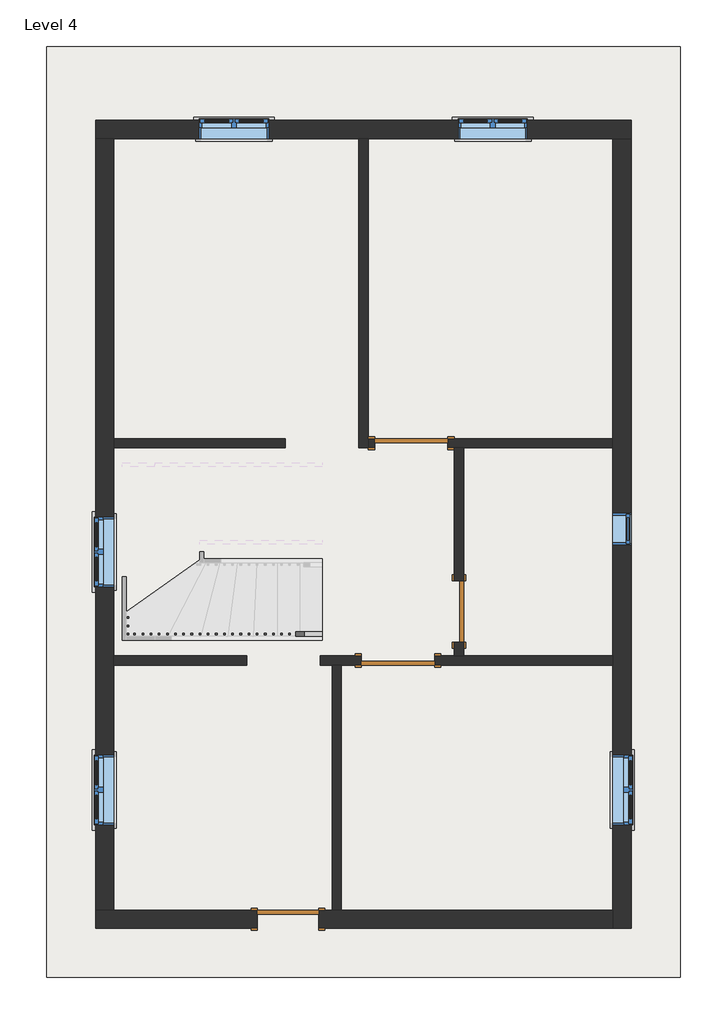
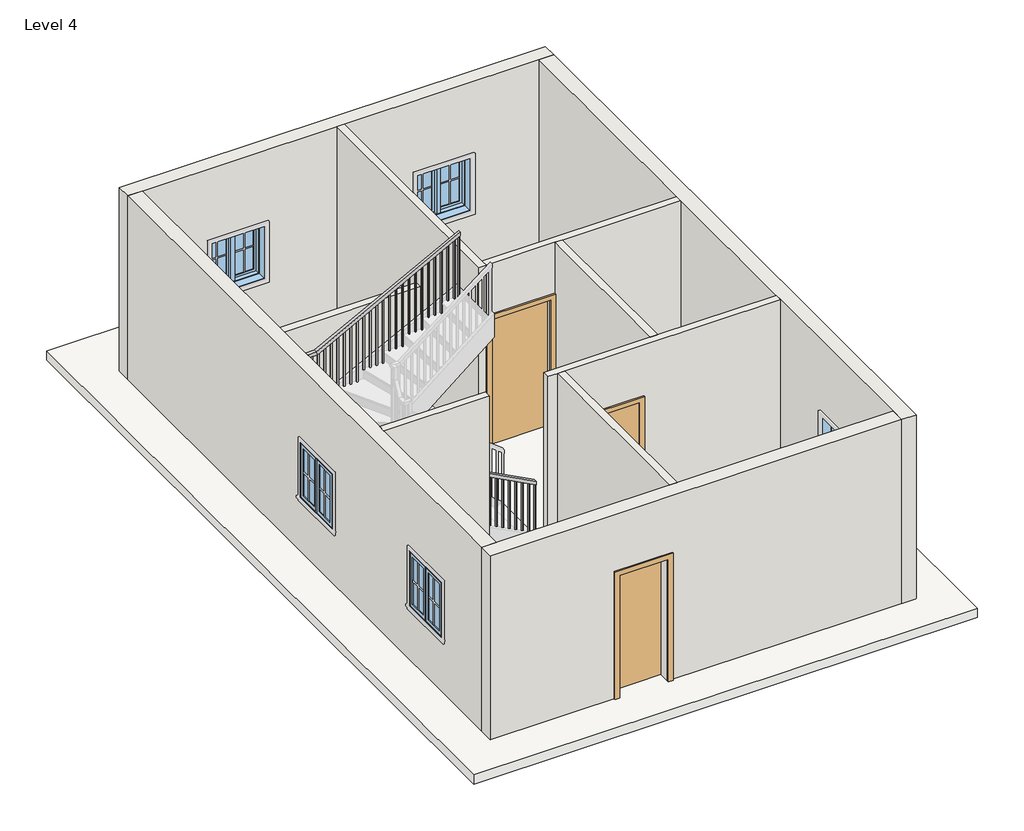
# One storey, part 1 of 2: 11 walls, 6 windows, 4 doors, 1 railing, 1 roof.
"""IFC4 building model written with IfcOpenShell, lengths in millimetres."""

from ifc_helpers import new_model, si_unit, frame, origin, place, context, project, spatial, polyline, outline, extrude, faceted_brep, transform, mapped, element, save
from components import door_d8f5dbb5, door_85036156, door_305aa2a5, door_e5f9f3c4, window_aa618e30, window_339605e1

model = new_model("IFC4")

# Units and contexts
model_context = context("Model", 3, world=origin())
ifc_project = project(units=[si_unit("LENGTHUNIT", "METRE", prefix="MILLI")], contexts=[model_context])

# Site, building, storey
site = spatial("IfcSite", under=ifc_project)
building = spatial("IfcBuilding", under=site)
storey = spatial("IfcBuildingStorey", under=building, Name="Level 4", Elevation=6400.8)

# Doors
placement = place(None, origin())
door_shape = door_d8f5dbb5(model_context)
element("IfcDoor", 1, ObjectType="Single-Flush : 30\" x 80\"", at=placement, inside=storey, context=model_context, shape_type="MappedRepresentation", body=[
    mapped(door_shape, transform((-82.2715692, -955.3070853, 6400.8), x_axis=(0.0, -1.0, 0.0), y_axis=(1.0, 0.0, 0.0), z_axis=(0.0, 0.0, 1.0))),
])
door_2_shape = door_85036156(model_context)
element("IfcDoor", 2, ObjectType="Single-Flush : 30\" x 80\"", at=placement, inside=storey, context=model_context, shape_type="MappedRepresentation", body=[
    mapped(door_2_shape, transform((-2212.5949167, -4784.3570853, 6400.8), x_axis=(-1.0, 0.0, 0.0), y_axis=(0.0, -1.0, 0.0), z_axis=(0.0, 0.0, 1.0))),
])
door_3_shape = door_305aa2a5(model_context)
element("IfcDoor", 3, ObjectType="Single-Flush : 36\" x 84\"", at=placement, inside=storey, context=model_context, shape_type="MappedRepresentation", body=[
    mapped(door_3_shape, transform((-677.5332429, 1140.1929147, 6400.8), x_axis=(-1.0, 0.0, 0.0), y_axis=(0.0, -1.0, 0.0), z_axis=(0.0, 0.0, 1.0))),
])
door_4_shape = door_e5f9f3c4(model_context)
element("IfcDoor", 4, ObjectType="Single-Flush : 36\" x 84\"", at=placement, inside=storey, context=model_context, shape_type="MappedRepresentation", body=[
    mapped(door_4_shape, transform((-842.6332429, -1564.9070853, 6400.8), x_axis=(-1.0, 0.0, 0.0), y_axis=(0.0, -1.0, 0.0), z_axis=(0.0, 0.0, 1.0))),
])

# Railing
element("IfcRailing", 5, ObjectType="Handrail - Rectangular", at=placement, inside=storey, context=model_context, shape_type="SolidModel", body=[
    faceted_brep([(-1783.4132248, -1260.1070853, 7484.5333333), (-1783.4132248, -1260.1070853, 7427.0742652), (-1783.4132248, -1209.3070853, 7427.0742652), (-1783.4132248, -1209.3070853, 7484.5333333), (-4041.1382869, -1260.1070853, 8677.8239201), (-4053.7373514, -1260.1070853, 8627.0239201), (-4053.7373514, -1209.3070853, 8627.0239201), (-4041.1382869, -1209.3070853, 8677.8239201), (-4225.5449167, -1260.1070853, 8677.8239201), (-4225.5449167, -1260.1070853, 8627.0239201), (-4174.7449167, -1209.3070853, 8627.0239201), (-4174.7449167, -1209.3070853, 8677.8239201), (-4225.5449167, -972.7952032, 8677.8239201), (-4225.5449167, -964.8446271, 8627.0239201), (-4174.7449167, -964.8446271, 8627.0239201), (-4174.7449167, -972.7952032, 8677.8239201), (-4225.5449167, 560.7810325, 9169.9094132), (-4225.5449167, 568.7316087, 9119.1094132), (-4174.7449167, 568.7316087, 9119.1094132), (-4174.7449167, 560.7810325, 9169.9094132), (-4225.5449167, 848.0929147, 9169.9094132), (-4225.5449167, 848.0929147, 9119.1094132), (-4174.7449167, 797.2929147, 9119.1094132), (-4174.7449167, 797.2929147, 9169.9094132), (-4041.1382869, 848.0929147, 9169.9094132), (-4028.5392223, 848.0929147, 9119.1094132), (-4028.5392223, 797.2929147, 9119.1094132), (-4041.1382869, 797.2929147, 9169.9094132), (-1783.4132248, 848.0929147, 10363.2), (-1783.4132248, 797.2929147, 10363.2), (-1783.4132248, 797.2929147, 10305.7409318), (-1783.4132248, 848.0929147, 10305.7409318)], [[[0, 1, 2, 3]], [[1, 0, 4, 5]], [[2, 1, 5, 6]], [[3, 2, 6, 7]], [[0, 3, 7, 4]], [[5, 4, 8, 9]], [[6, 5, 9, 10]], [[7, 6, 10, 11]], [[4, 7, 11, 8]], [[9, 8, 12, 13]], [[10, 9, 13, 14]], [[11, 10, 14, 15]], [[8, 11, 15, 12]], [[13, 12, 16, 17]], [[14, 13, 17, 18]], [[15, 14, 18, 19]], [[12, 15, 19, 16]], [[17, 16, 20, 21]], [[18, 17, 21, 22]], [[19, 18, 22, 23]], [[16, 19, 23, 20]], [[21, 20, 24, 25]], [[22, 21, 25, 26]], [[23, 22, 26, 27]], [[20, 23, 27, 24]], [[28, 29, 30, 31]], [[25, 24, 28, 31]], [[26, 25, 31, 30]], [[27, 26, 30, 29]], [[24, 27, 29, 28]]]),
    extrude(outline(polyline([(10258.4597858, -1872.8699167), (9279.4666667, -1872.8699167), (9279.4666667, -1853.8199167), (10268.5284102, -1853.8199167), (10258.4597858, -1872.8699167)])), frame((0.0, 813.1679147, 0.0), z_axis=(0.0, 1.0, 0.0), x_axis=(0.0, 0.0, 1.0)), (0.0, 0.0, 1.0), 19.05),
    extrude(outline(polyline([(10204.7604556, -1974.4699167), (9279.4666667, -1974.4699167), (9279.4666667, -1955.4199167), (10214.82908, -1955.4199167), (10204.7604556, -1974.4699167)])), frame((0.0, 813.1679147, 0.0), z_axis=(0.0, 1.0, 0.0), x_axis=(0.0, 0.0, 1.0)), (0.0, 0.0, 1.0), 19.05),
    extrude(outline(polyline([(10151.0611254, -2076.0699167), (9110.1333333, -2076.0699167), (9110.1333333, -2057.0199167), (10161.1297498, -2057.0199167), (10151.0611254, -2076.0699167)])), frame((0.0, 813.1679147, 0.0), z_axis=(0.0, 1.0, 0.0), x_axis=(0.0, 0.0, 1.0)), (0.0, 0.0, 1.0), 19.05),
    extrude(outline(polyline([(10097.3617952, -2177.6699167), (9110.1333333, -2177.6699167), (9110.1333333, -2158.6199167), (10107.4304196, -2158.6199167), (10097.3617952, -2177.6699167)])), frame((0.0, 813.1679147, 0.0), z_axis=(0.0, 1.0, 0.0), x_axis=(0.0, 0.0, 1.0)), (0.0, 0.0, 1.0), 19.05),
    extrude(outline(polyline([(10043.662465, -2279.2699167), (9110.1333333, -2279.2699167), (9110.1333333, -2260.2199167), (10053.7310894, -2260.2199167), (10043.662465, -2279.2699167)])), frame((0.0, 813.1679147, 0.0), z_axis=(0.0, 1.0, 0.0), x_axis=(0.0, 0.0, 1.0)), (0.0, 0.0, 1.0), 19.05),
    extrude(outline(polyline([(9989.9631348, -2380.8699167), (8940.8, -2380.8699167), (8940.8, -2361.8199167), (10000.0317592, -2361.8199167), (9989.9631348, -2380.8699167)])), frame((0.0, 813.1679147, 0.0), z_axis=(0.0, 1.0, 0.0), x_axis=(0.0, 0.0, 1.0)), (0.0, 0.0, 1.0), 19.05),
    extrude(outline(polyline([(9936.2638046, -2482.4699167), (8940.8, -2482.4699167), (8940.8, -2463.4199167), (9946.332429, -2463.4199167), (9936.2638046, -2482.4699167)])), frame((0.0, 813.1679147, 0.0), z_axis=(0.0, 1.0, 0.0), x_axis=(0.0, 0.0, 1.0)), (0.0, 0.0, 1.0), 19.05),
    extrude(outline(polyline([(9882.5644744, -2584.0699167), (8940.8, -2584.0699167), (8940.8, -2565.0199167), (9892.6330988, -2565.0199167), (9882.5644744, -2584.0699167)])), frame((0.0, 813.1679147, 0.0), z_axis=(0.0, 1.0, 0.0), x_axis=(0.0, 0.0, 1.0)), (0.0, 0.0, 1.0), 19.05),
    extrude(outline(polyline([(9828.8651442, -2685.6699167), (8771.4666667, -2685.6699167), (8771.4666667, -2666.6199167), (9838.9337686, -2666.6199167), (9828.8651442, -2685.6699167)])), frame((0.0, 813.1679147, 0.0), z_axis=(0.0, 1.0, 0.0), x_axis=(0.0, 0.0, 1.0)), (0.0, 0.0, 1.0), 19.05),
    extrude(outline(polyline([(9775.165814, -2787.2699167), (8771.4666667, -2787.2699167), (8771.4666667, -2768.2199167), (9785.2344384, -2768.2199167), (9775.165814, -2787.2699167)])), frame((0.0, 813.1679147, 0.0), z_axis=(0.0, 1.0, 0.0), x_axis=(0.0, 0.0, 1.0)), (0.0, 0.0, 1.0), 19.05),
    extrude(outline(polyline([(9721.4664838, -2888.8699167), (8771.4666667, -2888.8699167), (8771.4666667, -2869.8199167), (9731.5351082, -2869.8199167), (9721.4664838, -2888.8699167)])), frame((0.0, 813.1679147, 0.0), z_axis=(0.0, 1.0, 0.0), x_axis=(0.0, 0.0, 1.0)), (0.0, 0.0, 1.0), 19.05),
    extrude(outline(polyline([(9667.7671536, -2990.4699167), (8602.1333333, -2990.4699167), (8602.1333333, -2971.4199167), (9677.835778, -2971.4199167), (9667.7671536, -2990.4699167)])), frame((0.0, 813.1679147, 0.0), z_axis=(0.0, 1.0, 0.0), x_axis=(0.0, 0.0, 1.0)), (0.0, 0.0, 1.0), 19.05),
    extrude(outline(polyline([(9614.0678234, -3092.0699167), (8602.1333333, -3092.0699167), (8602.1333333, -3073.0199167), (9624.1364478, -3073.0199167), (9614.0678234, -3092.0699167)])), frame((0.0, 813.1679147, 0.0), z_axis=(0.0, 1.0, 0.0), x_axis=(0.0, 0.0, 1.0)), (0.0, 0.0, 1.0), 19.05),
    extrude(outline(polyline([(9560.3684932, -3193.6699167), (8602.1333333, -3193.6699167), (8602.1333333, -3174.6199167), (9570.4371176, -3174.6199167), (9560.3684932, -3193.6699167)])), frame((0.0, 813.1679147, 0.0), z_axis=(0.0, 1.0, 0.0), x_axis=(0.0, 0.0, 1.0)), (0.0, 0.0, 1.0), 19.05),
    extrude(outline(polyline([(9506.669163, -3295.2699167), (8602.1333333, -3295.2699167), (8602.1333333, -3276.2199167), (9516.7377874, -3276.2199167), (9506.669163, -3295.2699167)])), frame((0.0, 813.1679147, 0.0), z_axis=(0.0, 1.0, 0.0), x_axis=(0.0, 0.0, 1.0)), (0.0, 0.0, 1.0), 19.05),
    extrude(outline(polyline([(9452.9698328, -3396.8699167), (8432.8, -3396.8699167), (8432.8, -3377.8199167), (9463.0384572, -3377.8199167), (9452.9698328, -3396.8699167)])), frame((0.0, 813.1679147, 0.0), z_axis=(0.0, 1.0, 0.0), x_axis=(0.0, 0.0, 1.0)), (0.0, 0.0, 1.0), 19.05),
    extrude(outline(polyline([(9399.2705026, -3498.4699167), (8432.8, -3498.4699167), (8432.8, -3479.4199167), (9409.339127, -3479.4199167), (9399.2705026, -3498.4699167)])), frame((0.0, 813.1679147, 0.0), z_axis=(0.0, 1.0, 0.0), x_axis=(0.0, 0.0, 1.0)), (0.0, 0.0, 1.0), 19.05),
    extrude(outline(polyline([(9345.5711724, -3600.0699167), (8432.8, -3600.0699167), (8432.8, -3581.0199167), (9355.6397968, -3581.0199167), (9345.5711724, -3600.0699167)])), frame((0.0, 813.1679147, 0.0), z_axis=(0.0, 1.0, 0.0), x_axis=(0.0, 0.0, 1.0)), (0.0, 0.0, 1.0), 19.05),
    extrude(outline(polyline([(9291.8718422, -3701.6699167), (8432.8, -3701.6699167), (8432.8, -3682.6199167), (9301.9404666, -3682.6199167), (9291.8718422, -3701.6699167)])), frame((0.0, 813.1679147, 0.0), z_axis=(0.0, 1.0, 0.0), x_axis=(0.0, 0.0, 1.0)), (0.0, 0.0, 1.0), 19.05),
    extrude(outline(polyline([(9238.172512, -3803.2699167), (8263.4666667, -3803.2699167), (8263.4666667, -3784.2199167), (9248.2411364, -3784.2199167), (9238.172512, -3803.2699167)])), frame((0.0, 813.1679147, 0.0), z_axis=(0.0, 1.0, 0.0), x_axis=(0.0, 0.0, 1.0)), (0.0, 0.0, 1.0), 19.05),
    extrude(outline(polyline([(9184.4731818, -3904.8699167), (8263.4666667, -3904.8699167), (8263.4666667, -3885.8199167), (9194.5418062, -3885.8199167), (9184.4731818, -3904.8699167)])), frame((0.0, 813.1679147, 0.0), z_axis=(0.0, 1.0, 0.0), x_axis=(0.0, 0.0, 1.0)), (0.0, 0.0, 1.0), 19.05),
    extrude(outline(polyline([(9130.7738516, -4006.4699167), (8263.4666667, -4006.4699167), (8263.4666667, -3987.4199167), (9140.842476, -3987.4199167), (9130.7738516, -4006.4699167)])), frame((0.0, 813.1679147, 0.0), z_axis=(0.0, 1.0, 0.0), x_axis=(0.0, 0.0, 1.0)), (0.0, 0.0, 1.0), 19.05),
    extrude(outline(polyline([(-4108.0699167, 832.2179147), (-4089.0199167, 832.2179147), (-4089.0199167, 813.1679147), (-4108.0699167, 813.1679147), (-4108.0699167, 832.2179147)])), frame((0.0, 0.0, 8263.4666667), z_axis=(0.0, 0.0, 1.0), x_axis=(1.0, 0.0, 0.0)), (0.0, 0.0, 1.0), 855.6427466),
    extrude(outline(polyline([(-4209.6699167, 787.7679147), (-4209.6699167, 806.8179147), (-4190.6199167, 806.8179147), (-4190.6199167, 787.7679147), (-4209.6699167, 787.7679147)])), frame((0.0, 0.0, 8263.4666667), z_axis=(0.0, 0.0, 1.0), x_axis=(1.0, 0.0, 0.0)), (0.0, 0.0, 1.0), 855.6427466),
    extrude(outline(polyline([(-4209.6699167, 686.1679147), (-4209.6699167, 705.2179147), (-4190.6199167, 705.2179147), (-4190.6199167, 686.1679147), (-4209.6699167, 686.1679147)])), frame((0.0, 0.0, 8263.4666667), z_axis=(0.0, 0.0, 1.0), x_axis=(1.0, 0.0, 0.0)), (0.0, 0.0, 1.0), 855.6427466),
    extrude(outline(polyline([(-4209.6699167, 584.5679147), (-4209.6699167, 603.6179147), (-4190.6199167, 603.6179147), (-4190.6199167, 584.5679147), (-4209.6699167, 584.5679147)])), frame((0.0, 0.0, 8263.4666667), z_axis=(0.0, 0.0, 1.0), x_axis=(1.0, 0.0, 0.0)), (0.0, 0.0, 1.0), 855.6427466),
    extrude(outline(polyline([(502.0179147, 9097.7026907), (502.0179147, 8094.1333333), (482.9679147, 8094.1333333), (482.9679147, 9091.5900316), (502.0179147, 9097.7026907)])), frame((-4209.6699167, 0.0, 0.0), z_axis=(1.0, 0.0, 0.0), x_axis=(0.0, 1.0, 0.0)), (0.0, 0.0, 1.0), 19.05),
    extrude(outline(polyline([(400.4179147, 9065.1018425), (400.4179147, 8094.1333333), (381.3679147, 8094.1333333), (381.3679147, 9058.9891834), (400.4179147, 9065.1018425)])), frame((-4209.6699167, 0.0, 0.0), z_axis=(1.0, 0.0, 0.0), x_axis=(0.0, 1.0, 0.0)), (0.0, 0.0, 1.0), 19.05),
    extrude(outline(polyline([(298.8179147, 9032.5009942), (298.8179147, 8094.1333333), (279.7679147, 8094.1333333), (279.7679147, 9026.3883352), (298.8179147, 9032.5009942)])), frame((-4209.6699167, 0.0, 0.0), z_axis=(1.0, 0.0, 0.0), x_axis=(0.0, 1.0, 0.0)), (0.0, 0.0, 1.0), 19.05),
    extrude(outline(polyline([(197.2179147, 8999.900146), (197.2179147, 8094.1333333), (178.1679147, 8094.1333333), (178.1679147, 8993.787487), (197.2179147, 8999.900146)])), frame((-4209.6699167, 0.0, 0.0), z_axis=(1.0, 0.0, 0.0), x_axis=(0.0, 1.0, 0.0)), (0.0, 0.0, 1.0), 19.05),
    extrude(outline(polyline([(95.6179147, 8967.2992978), (95.6179147, 8094.1333333), (76.5679147, 8094.1333333), (76.5679147, 8961.1866387), (95.6179147, 8967.2992978)])), frame((-4209.6699167, 0.0, 0.0), z_axis=(1.0, 0.0, 0.0), x_axis=(0.0, 1.0, 0.0)), (0.0, 0.0, 1.0), 19.05),
    extrude(outline(polyline([(-5.9820853, 8934.6984495), (-5.9820853, 7924.8), (-25.0320853, 7924.8), (-25.0320853, 8928.5857905), (-5.9820853, 8934.6984495)])), frame((-4209.6699167, 0.0, 0.0), z_axis=(1.0, 0.0, 0.0), x_axis=(0.0, 1.0, 0.0)), (0.0, 0.0, 1.0), 19.05),
    extrude(outline(polyline([(-107.5820853, 8902.0976013), (-107.5820853, 7924.8), (-126.6320853, 7924.8), (-126.6320853, 8895.9849423), (-107.5820853, 8902.0976013)])), frame((-4209.6699167, 0.0, 0.0), z_axis=(1.0, 0.0, 0.0), x_axis=(0.0, 1.0, 0.0)), (0.0, 0.0, 1.0), 19.05),
    extrude(outline(polyline([(-209.1820853, 8869.4967531), (-209.1820853, 7924.8), (-228.2320853, 7924.8), (-228.2320853, 8863.384094), (-209.1820853, 8869.4967531)])), frame((-4209.6699167, 0.0, 0.0), z_axis=(1.0, 0.0, 0.0), x_axis=(0.0, 1.0, 0.0)), (0.0, 0.0, 1.0), 19.05),
    extrude(outline(polyline([(-310.7820853, 8836.8959049), (-310.7820853, 7924.8), (-329.8320853, 7924.8), (-329.8320853, 8830.7832458), (-310.7820853, 8836.8959049)])), frame((-4209.6699167, 0.0, 0.0), z_axis=(1.0, 0.0, 0.0), x_axis=(0.0, 1.0, 0.0)), (0.0, 0.0, 1.0), 19.05),
    extrude(outline(polyline([(-412.3820853, 8804.2950566), (-412.3820853, 7924.8), (-431.4320853, 7924.8), (-431.4320853, 8798.1823976), (-412.3820853, 8804.2950566)])), frame((-4209.6699167, 0.0, 0.0), z_axis=(1.0, 0.0, 0.0), x_axis=(0.0, 1.0, 0.0)), (0.0, 0.0, 1.0), 19.05),
    extrude(outline(polyline([(-513.9820853, 8771.6942084), (-513.9820853, 7755.4666667), (-533.0320853, 7755.4666667), (-533.0320853, 8765.5815494), (-513.9820853, 8771.6942084)])), frame((-4209.6699167, 0.0, 0.0), z_axis=(1.0, 0.0, 0.0), x_axis=(0.0, 1.0, 0.0)), (0.0, 0.0, 1.0), 19.05),
    extrude(outline(polyline([(-615.5820853, 8739.0933602), (-615.5820853, 7755.4666667), (-634.6320853, 7755.4666667), (-634.6320853, 8732.9807011), (-615.5820853, 8739.0933602)])), frame((-4209.6699167, 0.0, 0.0), z_axis=(1.0, 0.0, 0.0), x_axis=(0.0, 1.0, 0.0)), (0.0, 0.0, 1.0), 19.05),
    extrude(outline(polyline([(-717.1820853, 8706.492512), (-717.1820853, 7755.4666667), (-736.2320853, 7755.4666667), (-736.2320853, 8700.3798529), (-717.1820853, 8706.492512)])), frame((-4209.6699167, 0.0, 0.0), z_axis=(1.0, 0.0, 0.0), x_axis=(0.0, 1.0, 0.0)), (0.0, 0.0, 1.0), 19.05),
    extrude(outline(polyline([(-818.7820853, 8673.8916637), (-818.7820853, 7755.4666667), (-837.8320853, 7755.4666667), (-837.8320853, 8667.7790047), (-818.7820853, 8673.8916637)])), frame((-4209.6699167, 0.0, 0.0), z_axis=(1.0, 0.0, 0.0), x_axis=(0.0, 1.0, 0.0)), (0.0, 0.0, 1.0), 19.05),
    extrude(outline(polyline([(-920.3820853, 8641.2908155), (-920.3820853, 7755.4666667), (-939.4320853, 7755.4666667), (-939.4320853, 8635.1781565), (-920.3820853, 8641.2908155)])), frame((-4209.6699167, 0.0, 0.0), z_axis=(1.0, 0.0, 0.0), x_axis=(0.0, 1.0, 0.0)), (0.0, 0.0, 1.0), 19.05),
    extrude(outline(polyline([(-4209.6699167, -1041.0320853), (-4209.6699167, -1021.9820853), (-4190.6199167, -1021.9820853), (-4190.6199167, -1041.0320853), (-4209.6699167, -1041.0320853)])), frame((0.0, 0.0, 7586.1333333), z_axis=(0.0, 0.0, 1.0), x_axis=(1.0, 0.0, 0.0)), (0.0, 0.0, 1.0), 1040.8905868),
    extrude(outline(polyline([(-4209.6699167, -1142.6320853), (-4209.6699167, -1123.5820853), (-4190.6199167, -1123.5820853), (-4190.6199167, -1142.6320853), (-4209.6699167, -1142.6320853)])), frame((0.0, 0.0, 7586.1333333), z_axis=(0.0, 0.0, 1.0), x_axis=(1.0, 0.0, 0.0)), (0.0, 0.0, 1.0), 1040.8905868),
    extrude(outline(polyline([(-4110.6882248, -1244.2320853), (-4129.7382248, -1244.2320853), (-4129.7382248, -1225.1820853), (-4110.6882248, -1225.1820853), (-4110.6882248, -1244.2320853)])), frame((0.0, 0.0, 7586.1333333), z_axis=(0.0, 0.0, 1.0), x_axis=(1.0, 0.0, 0.0)), (0.0, 0.0, 1.0), 1040.8905868),
    extrude(outline(polyline([(8613.4938418, -4028.1382248), (7586.1333333, -4028.1382248), (7586.1333333, -4009.0882248), (8603.4252174, -4009.0882248), (8613.4938418, -4028.1382248)])), frame((0.0, -1244.2320853, 0.0), z_axis=(0.0, 1.0, 0.0), x_axis=(0.0, 0.0, 1.0)), (0.0, 0.0, 1.0), 19.05),
    extrude(outline(polyline([(8559.7945116, -3926.5382248), (7586.1333333, -3926.5382248), (7586.1333333, -3907.4882248), (8549.7258872, -3907.4882248), (8559.7945116, -3926.5382248)])), frame((0.0, -1244.2320853, 0.0), z_axis=(0.0, 1.0, 0.0), x_axis=(0.0, 0.0, 1.0)), (0.0, 0.0, 1.0), 19.05),
    extrude(outline(polyline([(8506.0951814, -3824.9382248), (7586.1333333, -3824.9382248), (7586.1333333, -3805.8882248), (8496.026557, -3805.8882248), (8506.0951814, -3824.9382248)])), frame((0.0, -1244.2320853, 0.0), z_axis=(0.0, 1.0, 0.0), x_axis=(0.0, 0.0, 1.0)), (0.0, 0.0, 1.0), 19.05),
    extrude(outline(polyline([(8452.3958512, -3723.3382248), (7586.1333333, -3723.3382248), (7586.1333333, -3704.2882248), (8442.3272268, -3704.2882248), (8452.3958512, -3723.3382248)])), frame((0.0, -1244.2320853, 0.0), z_axis=(0.0, 1.0, 0.0), x_axis=(0.0, 0.0, 1.0)), (0.0, 0.0, 1.0), 19.05),
    extrude(outline(polyline([(8398.696521, -3621.7382248), (7416.8, -3621.7382248), (7416.8, -3602.6882248), (8388.6278966, -3602.6882248), (8398.696521, -3621.7382248)])), frame((0.0, -1244.2320853, 0.0), z_axis=(0.0, 1.0, 0.0), x_axis=(0.0, 0.0, 1.0)), (0.0, 0.0, 1.0), 19.05),
    extrude(outline(polyline([(8344.9971908, -3520.1382248), (7416.8, -3520.1382248), (7416.8, -3501.0882248), (8334.9285664, -3501.0882248), (8344.9971908, -3520.1382248)])), frame((0.0, -1244.2320853, 0.0), z_axis=(0.0, 1.0, 0.0), x_axis=(0.0, 0.0, 1.0)), (0.0, 0.0, 1.0), 19.05),
    extrude(outline(polyline([(8291.2978606, -3418.5382248), (7416.8, -3418.5382248), (7416.8, -3399.4882248), (8281.2292362, -3399.4882248), (8291.2978606, -3418.5382248)])), frame((0.0, -1244.2320853, 0.0), z_axis=(0.0, 1.0, 0.0), x_axis=(0.0, 0.0, 1.0)), (0.0, 0.0, 1.0), 19.05),
    extrude(outline(polyline([(8237.5985304, -3316.9382248), (7416.8, -3316.9382248), (7416.8, -3297.8882248), (8227.529906, -3297.8882248), (8237.5985304, -3316.9382248)])), frame((0.0, -1244.2320853, 0.0), z_axis=(0.0, 1.0, 0.0), x_axis=(0.0, 0.0, 1.0)), (0.0, 0.0, 1.0), 19.05),
    extrude(outline(polyline([(8183.8992002, -3215.3382248), (7247.4666667, -3215.3382248), (7247.4666667, -3196.2882248), (8173.8305758, -3196.2882248), (8183.8992002, -3215.3382248)])), frame((0.0, -1244.2320853, 0.0), z_axis=(0.0, 1.0, 0.0), x_axis=(0.0, 0.0, 1.0)), (0.0, 0.0, 1.0), 19.05),
    extrude(outline(polyline([(8130.19987, -3113.7382248), (7247.4666667, -3113.7382248), (7247.4666667, -3094.6882248), (8120.1312456, -3094.6882248), (8130.19987, -3113.7382248)])), frame((0.0, -1244.2320853, 0.0), z_axis=(0.0, 1.0, 0.0), x_axis=(0.0, 0.0, 1.0)), (0.0, 0.0, 1.0), 19.05),
    extrude(outline(polyline([(8076.5005398, -3012.1382248), (7247.4666667, -3012.1382248), (7247.4666667, -2993.0882248), (8066.4319154, -2993.0882248), (8076.5005398, -3012.1382248)])), frame((0.0, -1244.2320853, 0.0), z_axis=(0.0, 1.0, 0.0), x_axis=(0.0, 0.0, 1.0)), (0.0, 0.0, 1.0), 19.05),
    extrude(outline(polyline([(8022.8012096, -2910.5382248), (7078.1333333, -2910.5382248), (7078.1333333, -2891.4882248), (8012.7325852, -2891.4882248), (8022.8012096, -2910.5382248)])), frame((0.0, -1244.2320853, 0.0), z_axis=(0.0, 1.0, 0.0), x_axis=(0.0, 0.0, 1.0)), (0.0, 0.0, 1.0), 19.05),
    extrude(outline(polyline([(7969.1018794, -2808.9382248), (7078.1333333, -2808.9382248), (7078.1333333, -2789.8882248), (7959.033255, -2789.8882248), (7969.1018794, -2808.9382248)])), frame((0.0, -1244.2320853, 0.0), z_axis=(0.0, 1.0, 0.0), x_axis=(0.0, 0.0, 1.0)), (0.0, 0.0, 1.0), 19.05),
    extrude(outline(polyline([(7915.4025492, -2707.3382248), (7078.1333333, -2707.3382248), (7078.1333333, -2688.2882248), (7905.3339248, -2688.2882248), (7915.4025492, -2707.3382248)])), frame((0.0, -1244.2320853, 0.0), z_axis=(0.0, 1.0, 0.0), x_axis=(0.0, 0.0, 1.0)), (0.0, 0.0, 1.0), 19.05),
    extrude(outline(polyline([(7861.703219, -2605.7382248), (6908.8, -2605.7382248), (6908.8, -2586.6882248), (7851.6345946, -2586.6882248), (7861.703219, -2605.7382248)])), frame((0.0, -1244.2320853, 0.0), z_axis=(0.0, 1.0, 0.0), x_axis=(0.0, 0.0, 1.0)), (0.0, 0.0, 1.0), 19.05),
    extrude(outline(polyline([(7808.0038888, -2504.1382248), (6908.8, -2504.1382248), (6908.8, -2485.0882248), (7797.9352644, -2485.0882248), (7808.0038888, -2504.1382248)])), frame((0.0, -1244.2320853, 0.0), z_axis=(0.0, 1.0, 0.0), x_axis=(0.0, 0.0, 1.0)), (0.0, 0.0, 1.0), 19.05),
    extrude(outline(polyline([(7754.3045586, -2402.5382248), (6908.8, -2402.5382248), (6908.8, -2383.4882248), (7744.2359342, -2383.4882248), (7754.3045586, -2402.5382248)])), frame((0.0, -1244.2320853, 0.0), z_axis=(0.0, 1.0, 0.0), x_axis=(0.0, 0.0, 1.0)), (0.0, 0.0, 1.0), 19.05),
    extrude(outline(polyline([(7700.6052284, -2300.9382248), (6739.4666667, -2300.9382248), (6739.4666667, -2281.8882248), (7690.536604, -2281.8882248), (7700.6052284, -2300.9382248)])), frame((0.0, -1244.2320853, 0.0), z_axis=(0.0, 1.0, 0.0), x_axis=(0.0, 0.0, 1.0)), (0.0, 0.0, 1.0), 19.05),
    extrude(outline(polyline([(7646.9058982, -2199.3382248), (6739.4666667, -2199.3382248), (6739.4666667, -2180.2882248), (7636.8372738, -2180.2882248), (7646.9058982, -2199.3382248)])), frame((0.0, -1244.2320853, 0.0), z_axis=(0.0, 1.0, 0.0), x_axis=(0.0, 0.0, 1.0)), (0.0, 0.0, 1.0), 19.05),
    extrude(outline(polyline([(7593.206568, -2097.7382248), (6739.4666667, -2097.7382248), (6739.4666667, -2078.6882248), (7583.1379436, -2078.6882248), (7593.206568, -2097.7382248)])), frame((0.0, -1244.2320853, 0.0), z_axis=(0.0, 1.0, 0.0), x_axis=(0.0, 0.0, 1.0)), (0.0, 0.0, 1.0), 19.05),
    extrude(outline(polyline([(7539.5072378, -1996.1382248), (6570.1333333, -1996.1382248), (6570.1333333, -1977.0882248), (7529.4386134, -1977.0882248), (7539.5072378, -1996.1382248)])), frame((0.0, -1244.2320853, 0.0), z_axis=(0.0, 1.0, 0.0), x_axis=(0.0, 0.0, 1.0)), (0.0, 0.0, 1.0), 19.05),
    extrude(outline(polyline([(7485.8079076, -1894.5382248), (6570.1333333, -1894.5382248), (6570.1333333, -1875.4882248), (7475.7392831, -1875.4882248), (7485.8079076, -1894.5382248)])), frame((0.0, -1244.2320853, 0.0), z_axis=(0.0, 1.0, 0.0), x_axis=(0.0, 0.0, 1.0)), (0.0, 0.0, 1.0), 19.05),
    extrude(outline(polyline([(-4209.6699167, 813.1679147), (-4209.6699167, 832.2179147), (-4190.6199167, 832.2179147), (-4190.6199167, 813.1679147), (-4209.6699167, 813.1679147)])), frame((0.0, 0.0, 8263.4666667), z_axis=(0.0, 0.0, 1.0), x_axis=(1.0, 0.0, 0.0)), (0.0, 0.0, 1.0), 855.6427466),
    extrude(outline(polyline([(-4190.6199167, -1244.2320853), (-4209.6699167, -1244.2320853), (-4209.6699167, -1225.1820853), (-4190.6199167, -1225.1820853), (-4190.6199167, -1244.2320853)])), frame((0.0, 0.0, 7586.1333333), z_axis=(0.0, 0.0, 1.0), x_axis=(1.0, 0.0, 0.0)), (0.0, 0.0, 1.0), 1040.8905868),
    extrude(outline(polyline([(10295.6723074, -1802.4632248), (9279.4666667, -1802.4632248), (9279.4666667, -1783.4132248), (10305.7409318, -1783.4132248), (10295.6723074, -1802.4632248)])), frame((0.0, 813.1679147, 0.0), z_axis=(0.0, 1.0, 0.0), x_axis=(0.0, 0.0, 1.0)), (0.0, 0.0, 1.0), 19.05),
    extrude(outline(polyline([(7437.1428896, -1802.4632248), (6570.1333333, -1802.4632248), (6570.1333333, -1783.4132248), (7427.0742652, -1783.4132248), (7437.1428896, -1802.4632248)])), frame((0.0, -1244.2320853, 0.0), z_axis=(0.0, 1.0, 0.0), x_axis=(0.0, 0.0, 1.0)), (0.0, 0.0, 1.0), 19.05),
])

# Roof
element("IfcRoof", 6, ObjectType="Generic - 12\"", at=placement, inside=storey, context=model_context, shape_type="SweptSolid", body=[
    extrude(outline(polyline([(-5216.1449167, 6076.3773594), (2670.5550833, 6076.3773594), (2670.5550833, -5508.2570853), (-5216.1449167, -5508.2570853), (-5216.1449167, 6076.3773594)])), frame((0.0, 0.0, 6248.4), z_axis=(0.0, 0.0, 1.0), x_axis=(1.0, 0.0, 0.0)), (0.0, 0.0, 1.0), 152.4),
])

# Walls
element("IfcWall", 7, ObjectType="WALL4.5\"", at=placement, inside=storey, context=model_context, shape_type="Brep", body=[
    faceted_brep([(-1329.9449167, 4931.1429147, 6400.8), (-1329.9449167, 1083.0429147, 6400.8), (-1329.9449167, 1083.0429147, 9448.8), (-1329.9449167, 4931.1429147, 9448.8), (-1215.6449167, 4931.1429147, 6400.8), (-1215.6449167, 4931.1429147, 9448.8), (-1215.6449167, 1197.3429147, 9448.8), (-1215.6449167, 1083.0429147, 9448.8), (-1215.6449167, 1083.0429147, 6400.8), (-1215.6449167, 1197.3429147, 6400.8)], [[[0, 1, 2, 3]], [[4, 5, 6, 7, 8, 9]], [[1, 0, 4, 9, 8]], [[0, 3, 5, 4]], [[2, 1, 8, 7]], [[3, 2, 7, 6, 5]]]),
])
element("IfcWall", 8, ObjectType="WALL4.5\"", at=placement, inside=storey, context=model_context, shape_type="Brep", body=[
    faceted_brep([(-1215.6449167, 1083.0429147, 6400.8), (-1134.7332429, 1083.0429147, 6400.8), (-1134.7332429, 1083.0429147, 8534.4), (-220.3332429, 1083.0429147, 8534.4), (-220.3332429, 1083.0429147, 6400.8), (-139.4215692, 1083.0429147, 6400.8), (-25.1215692, 1083.0429147, 6400.8), (1832.3550833, 1083.0429147, 6400.8), (1832.3550833, 1083.0429147, 9448.8), (-25.1215692, 1083.0429147, 9448.8), (-139.4215692, 1083.0429147, 9448.8), (-1215.6449167, 1083.0429147, 9448.8), (-1134.7332429, 1197.3429147, 8534.4), (-1134.7332429, 1197.3429147, 6400.8), (-1215.6449167, 1197.3429147, 6400.8), (-1215.6449167, 1197.3429147, 9448.8), (1832.3550833, 1197.3429147, 9448.8), (1832.3550833, 1197.3429147, 6400.8), (-220.3332429, 1197.3429147, 6400.8), (-220.3332429, 1197.3429147, 8534.4)], [[[0, 1, 2, 3, 4, 5, 6, 7, 8, 9, 10, 11]], [[12, 13, 14, 15, 16, 17, 18, 19]], [[18, 17, 7, 6, 5, 4]], [[14, 13, 1, 0]], [[0, 11, 15, 14]], [[8, 7, 17, 16]], [[2, 1, 13, 12]], [[3, 2, 12, 19]], [[4, 3, 19, 18]], [[11, 10, 9, 8, 16, 15]]]),
])
element("IfcWall", 9, ObjectType="WALL4.5\"", at=placement, inside=storey, context=model_context, shape_type="SweptSolid", body=[
    extrude(outline(polyline([(-2244.3449167, 1083.0429147), (-4377.9449167, 1083.0429147), (-4377.9449167, 1197.3429147), (-2244.3449167, 1197.3429147), (-2244.3449167, 1083.0429147)])), frame((0.0, 0.0, 6400.8), z_axis=(0.0, 0.0, 1.0), x_axis=(1.0, 0.0, 0.0)), (0.0, 0.0, 1.0), 3048.0),
])
element("IfcWall", 10, ObjectType="WALL4.5\"", at=placement, inside=storey, context=model_context, shape_type="SweptSolid", body=[
    extrude(outline(polyline([(-1336.3070853, 8432.8), (-1336.3070853, 6400.8), (-1507.7570853, 6400.8), (-1507.7570853, 9448.8), (1083.0429147, 9448.8), (1083.0429147, 6400.8), (-574.3070853, 6400.8), (-574.3070853, 8432.8), (-1336.3070853, 8432.8)])), frame((-139.4215692, 0.0, 0.0), z_axis=(1.0, 0.0, 0.0), x_axis=(0.0, 1.0, 0.0)), (0.0, 0.0, 1.0), 114.3),
])
element("IfcWall", 11, ObjectType="WALL4.5\"", at=placement, inside=storey, context=model_context, shape_type="SweptSolid", body=[
    extrude(outline(polyline([(-2726.9449167, -1622.0570853), (-4377.9449167, -1622.0570853), (-4377.9449167, -1507.7570853), (-2726.9449167, -1507.7570853), (-2726.9449167, -1622.0570853)])), frame((0.0, 0.0, 6400.8), z_axis=(0.0, 0.0, 1.0), x_axis=(1.0, 0.0, 0.0)), (0.0, 0.0, 1.0), 3048.0),
])
element("IfcWall", 12, ObjectType="WALL4.5\"", at=placement, inside=storey, context=model_context, shape_type="Brep", body=[
    faceted_brep([(-1812.5449167, -1622.0570853, 6400.8), (-1660.1449167, -1622.0570853, 6400.8), (-1545.8449167, -1622.0570853, 6400.8), (-1299.8332429, -1622.0570853, 6400.8), (-1299.8332429, -1622.0570853, 8534.4), (-385.4332429, -1622.0570853, 8534.4), (-385.4332429, -1622.0570853, 6400.8), (1832.3550833, -1622.0570853, 6400.8), (1832.3550833, -1622.0570853, 9448.8), (-1545.8449167, -1622.0570853, 9448.8), (-1660.1449167, -1622.0570853, 9448.8), (-1812.5449167, -1622.0570853, 9448.8), (-1299.8332429, -1507.7570853, 8534.4), (-1299.8332429, -1507.7570853, 6400.8), (-1812.5449167, -1507.7570853, 6400.8), (-1812.5449167, -1507.7570853, 9448.8), (-139.4215692, -1507.7570853, 9448.8), (-25.1215692, -1507.7570853, 9448.8), (1832.3550833, -1507.7570853, 9448.8), (1832.3550833, -1507.7570853, 6400.8), (-25.1215692, -1507.7570853, 6400.8), (-139.4215692, -1507.7570853, 6400.8), (-385.4332429, -1507.7570853, 6400.8), (-385.4332429, -1507.7570853, 8534.4)], [[[0, 1, 2, 3, 4, 5, 6, 7, 8, 9, 10, 11]], [[12, 13, 14, 15, 16, 17, 18, 19, 20, 21, 22, 23]], [[14, 13, 3, 2, 1, 0]], [[22, 21, 20, 19, 7, 6]], [[0, 11, 15, 14]], [[8, 7, 19, 18]], [[4, 3, 13, 12]], [[5, 4, 12, 23]], [[6, 5, 23, 22]], [[11, 10, 9, 8, 18, 17, 16, 15]]]),
])
element("IfcWall", 13, ObjectType="WALL4.5\"", at=placement, inside=storey, context=model_context, shape_type="SweptSolid", body=[
    extrude(outline(polyline([(-1660.1449167, -4670.0570853), (-1660.1449167, -1622.0570853), (-1545.8449167, -1622.0570853), (-1545.8449167, -4670.0570853), (-1660.1449167, -4670.0570853)])), frame((0.0, 0.0, 6400.8), z_axis=(0.0, 0.0, 1.0), x_axis=(1.0, 0.0, 0.0)), (0.0, 0.0, 1.0), 3048.0),
])
element("IfcWall", 14, ObjectType="WALL9\"", at=placement, inside=storey, context=model_context, shape_type="Brep", body=[
    faceted_brep([(-4606.5449167, 4931.1429147, 6400.8), (-4377.9449167, 4931.1429147, 6400.8), (-1329.9449167, 4931.1429147, 6400.8), (-1215.6449167, 4931.1429147, 6400.8), (1832.3550833, 4931.1429147, 6400.8), (2060.9550833, 4931.1429147, 6400.8), (2060.9550833, 4931.1429147, 9448.8), (1832.3550833, 4931.1429147, 9448.8), (-1215.6449167, 4931.1429147, 9448.8), (-1329.9449167, 4931.1429147, 9448.8), (-4377.9449167, 4931.1429147, 9448.8), (-4606.5449167, 4931.1429147, 9448.8), (-2450.7199167, 4931.1429147, 8229.6), (-2450.7199167, 4931.1429147, 7315.2), (-3314.3199167, 4931.1429147, 7315.2), (-3314.3199167, 4931.1429147, 8229.6), (768.7300833, 4931.1429147, 8229.6), (768.7300833, 4931.1429147, 7315.2), (-94.8699167, 4931.1429147, 7315.2), (-94.8699167, 4931.1429147, 8229.6), (-4606.5449167, 5159.7429147, 6400.8), (-4606.5449167, 5159.7429147, 9448.8), (2060.9550833, 5159.7429147, 9448.8), (2060.9550833, 5159.7429147, 6400.8), (-2450.7199167, 5159.7429147, 8229.6), (-3314.3199167, 5159.7429147, 8229.6), (-3314.3199167, 5159.7429147, 7315.2), (-2450.7199167, 5159.7429147, 7315.2), (768.7300833, 5159.7429147, 8229.6), (-94.8699167, 5159.7429147, 8229.6), (-94.8699167, 5159.7429147, 7315.2), (768.7300833, 5159.7429147, 7315.2)], [[[0, 1, 2, 3, 4, 5, 6, 7, 8, 9, 10, 11], [12, 13, 14, 15], [16, 17, 18, 19]], [[20, 21, 22, 23], [24, 25, 26, 27], [28, 29, 30, 31]], [[5, 4, 3, 2, 1, 0, 20, 23]], [[6, 5, 23, 22]], [[0, 11, 21, 20]], [[13, 12, 24, 27]], [[14, 13, 27, 26]], [[15, 14, 26, 25]], [[12, 15, 25, 24]], [[17, 16, 28, 31]], [[18, 17, 31, 30]], [[19, 18, 30, 29]], [[16, 19, 29, 28]], [[11, 10, 9, 8, 7, 6, 22, 21]]]),
])
element("IfcWall", 15, ObjectType="WALL9\"", at=placement, inside=storey, context=model_context, shape_type="Brep", body=[
    faceted_brep([(1832.3550833, 4931.1429147, 6400.8), (1832.3550833, 1197.3429147, 6400.8), (1832.3550833, 1083.0429147, 6400.8), (1832.3550833, -1507.7570853, 6400.8), (1832.3550833, -1622.0570853, 6400.8), (1832.3550833, -4670.0570853, 6400.8), (1832.3550833, -4898.6570853, 6400.8), (1832.3550833, -4898.6570853, 9448.8), (1832.3550833, -4670.0570853, 9448.8), (1832.3550833, -1622.0570853, 9448.8), (1832.3550833, -1507.7570853, 9448.8), (1832.3550833, 1083.0429147, 9448.8), (1832.3550833, 1197.3429147, 9448.8), (1832.3550833, 4931.1429147, 9448.8), (1832.3550833, -129.8070853, 7924.8), (1832.3550833, -129.8070853, 7315.2), (1832.3550833, 276.5929147, 7315.2), (1832.3550833, 276.5929147, 7924.8), (1832.3550833, -3606.4320853, 8229.6), (1832.3550833, -3606.4320853, 7315.2), (1832.3550833, -2742.8320853, 7315.2), (1832.3550833, -2742.8320853, 8229.6), (2060.9550833, 4931.1429147, 6400.8), (2060.9550833, 4931.1429147, 9448.8), (2060.9550833, -4898.6570853, 9448.8), (2060.9550833, -4898.6570853, 6400.8), (2060.9550833, -129.8070853, 7924.8), (2060.9550833, 276.5929147, 7924.8), (2060.9550833, 276.5929147, 7315.2), (2060.9550833, -129.8070853, 7315.2), (2060.9550833, -3606.4320853, 8229.6), (2060.9550833, -2742.8320853, 8229.6), (2060.9550833, -2742.8320853, 7315.2), (2060.9550833, -3606.4320853, 7315.2)], [[[0, 1, 2, 3, 4, 5, 6, 7, 8, 9, 10, 11, 12, 13], [14, 15, 16, 17], [18, 19, 20, 21]], [[22, 23, 24, 25], [26, 27, 28, 29], [30, 31, 32, 33]], [[6, 5, 4, 3, 2, 1, 0, 22, 25]], [[0, 13, 23, 22]], [[7, 6, 25, 24]], [[15, 14, 26, 29]], [[16, 15, 29, 28]], [[17, 16, 28, 27]], [[14, 17, 27, 26]], [[19, 18, 30, 33]], [[20, 19, 33, 32]], [[21, 20, 32, 31]], [[18, 21, 31, 30]], [[13, 12, 11, 10, 9, 8, 7, 24, 23]]]),
])
element("IfcWall", 16, ObjectType="WALL9\"", at=placement, inside=storey, context=model_context, shape_type="Brep", body=[
    faceted_brep([(-2593.5949167, -4670.0570853, 8432.8), (-2593.5949167, -4670.0570853, 6400.8), (-4377.9449167, -4670.0570853, 6400.8), (-4606.5449167, -4670.0570853, 6400.8), (-4606.5449167, -4670.0570853, 9448.8), (-4377.9449167, -4670.0570853, 9448.8), (-1660.1449167, -4670.0570853, 9448.8), (-1545.8449167, -4670.0570853, 9448.8), (1832.3550833, -4670.0570853, 9448.8), (1832.3550833, -4670.0570853, 6400.8), (-1545.8449167, -4670.0570853, 6400.8), (-1660.1449167, -4670.0570853, 6400.8), (-1831.5949167, -4670.0570853, 6400.8), (-1831.5949167, -4670.0570853, 8432.8), (-4606.5449167, -4898.6570853, 6400.8), (-2593.5949167, -4898.6570853, 6400.8), (-2593.5949167, -4898.6570853, 8432.8), (-1831.5949167, -4898.6570853, 8432.8), (-1831.5949167, -4898.6570853, 6400.8), (1832.3550833, -4898.6570853, 6400.8), (1832.3550833, -4898.6570853, 9448.8), (-4606.5449167, -4898.6570853, 9448.8)], [[[0, 1, 2, 3, 4, 5, 6, 7, 8, 9, 10, 11, 12, 13]], [[14, 15, 16, 17, 18, 19, 20, 21]], [[3, 2, 1, 15, 14]], [[12, 11, 10, 9, 19, 18]], [[9, 8, 20, 19]], [[4, 3, 14, 21]], [[16, 15, 1, 0]], [[17, 16, 0, 13]], [[18, 17, 13, 12]], [[8, 7, 6, 5, 4, 21, 20]]]),
])
element("IfcWall", 17, ObjectType="WALL9\"", at=placement, inside=storey, context=model_context, shape_type="Brep", body=[
    faceted_brep([(-4377.9449167, -4670.0570853, 6400.8), (-4377.9449167, -1622.0570853, 6400.8), (-4377.9449167, -1507.7570853, 6400.8), (-4377.9449167, 1083.0429147, 6400.8), (-4377.9449167, 1197.3429147, 6400.8), (-4377.9449167, 4931.1429147, 6400.8), (-4377.9449167, 4931.1429147, 9448.8), (-4377.9449167, 1197.3429147, 9448.8), (-4377.9449167, 1083.0429147, 9448.8), (-4377.9449167, -1507.7570853, 9448.8), (-4377.9449167, -1622.0570853, 9448.8), (-4377.9449167, -4670.0570853, 9448.8), (-4377.9449167, -2742.8320853, 8229.6), (-4377.9449167, -2742.8320853, 7315.2), (-4377.9449167, -3606.4320853, 7315.2), (-4377.9449167, -3606.4320853, 8229.6), (-4377.9449167, 219.4429147, 8229.6), (-4377.9449167, 219.4429147, 7315.2), (-4377.9449167, -644.1570853, 7315.2), (-4377.9449167, -644.1570853, 8229.6), (-4606.5449167, -4670.0570853, 6400.8), (-4606.5449167, -4670.0570853, 9448.8), (-4606.5449167, 4931.1429147, 9448.8), (-4606.5449167, 4931.1429147, 6400.8), (-4606.5449167, -2742.8320853, 8229.6), (-4606.5449167, -3606.4320853, 8229.6), (-4606.5449167, -3606.4320853, 7315.2), (-4606.5449167, -2742.8320853, 7315.2), (-4606.5449167, 219.4429147, 8229.6), (-4606.5449167, -644.1570853, 8229.6), (-4606.5449167, -644.1570853, 7315.2), (-4606.5449167, 219.4429147, 7315.2)], [[[0, 1, 2, 3, 4, 5, 6, 7, 8, 9, 10, 11], [12, 13, 14, 15], [16, 17, 18, 19]], [[20, 21, 22, 23], [24, 25, 26, 27], [28, 29, 30, 31]], [[5, 4, 3, 2, 1, 0, 20, 23]], [[0, 11, 21, 20]], [[6, 5, 23, 22]], [[13, 12, 24, 27]], [[14, 13, 27, 26]], [[15, 14, 26, 25]], [[12, 15, 25, 24]], [[17, 16, 28, 31]], [[18, 17, 31, 30]], [[19, 18, 30, 29]], [[16, 19, 29, 28]], [[11, 10, 9, 8, 7, 6, 22, 21]]]),
])

# Windows
window_shape = window_aa618e30(model_context)
element("IfcWindow", 18, ObjectType="Fixed : 16\" x 24\"", at=placement, inside=storey, context=model_context, shape_type="MappedRepresentation", body=[
    mapped(window_shape, transform((1946.6550833, 35.2929147, 6400.8), x_axis=(0.0, -1.0, 0.0), y_axis=(1.0, 0.0, 0.0), z_axis=(0.0, 0.0, 1.0))),
])
window_2_shape = window_339605e1(model_context)
element("IfcWindow", 19, ObjectType="Window-Casement-Double : 34\" x 36\"", at=placement, inside=storey, context=model_context, shape_type="MappedRepresentation", body=[
    mapped(window_2_shape, transform((-2882.5199167, 5045.4429147, 6400.8), x_axis=(1.0, 0.0, 0.0), y_axis=(0.0, 1.0, 0.0), z_axis=(0.0, 0.0, 1.0))),
])
element("IfcWindow", 20, ObjectType="Window-Casement-Double : 34\" x 36\"", at=placement, inside=storey, context=model_context, shape_type="MappedRepresentation", body=[
    mapped(window_2_shape, transform((336.9300833, 5045.4429147, 6400.8), x_axis=(1.0, 0.0, 0.0), y_axis=(0.0, 1.0, 0.0), z_axis=(0.0, 0.0, 1.0))),
])
element("IfcWindow", 21, ObjectType="Window-Casement-Double : 34\" x 36\"", at=placement, inside=storey, context=model_context, shape_type="MappedRepresentation", body=[
    mapped(window_2_shape, transform((1946.6550833, -3174.6320853, 6400.8), x_axis=(0.0, -1.0, 0.0), y_axis=(1.0, 0.0, 0.0), z_axis=(0.0, 0.0, 1.0))),
])
element("IfcWindow", 22, ObjectType="Window-Casement-Double : 34\" x 36\"", at=placement, inside=storey, context=model_context, shape_type="MappedRepresentation", body=[
    mapped(window_2_shape, transform((-4492.2449167, -3174.6320853, 6400.8), x_axis=(0.0, 1.0, 0.0), y_axis=(-1.0, 0.0, 0.0), z_axis=(0.0, 0.0, 1.0))),
])
element("IfcWindow", 23, ObjectType="Window-Casement-Double : 34\" x 36\"", at=placement, inside=storey, context=model_context, shape_type="MappedRepresentation", body=[
    mapped(window_2_shape, transform((-4492.2449167, -212.3570853, 6400.8), x_axis=(0.0, 1.0, 0.0), y_axis=(-1.0, 0.0, 0.0), z_axis=(0.0, 0.0, 1.0))),
])

save(model, "model.ifc")

# Revit data of these elements
# Type "Single-Flush : 30\" x 80\""
#   Type Mark = "5"
#   Construction Type Id = "MDOOR"
#   Assembly Code = "C1020"
#   Analytic Construction = "Metal"
#   Thickness = 0' - 2"
#   Heat Transfer Coefficient (U) = 0.651978 BTU/(h·ft²·°F)
#   Height = 6' - 8"
#   Trim Projection Ext = 0' - 1"
#   Trim Projection Int = 0' - 1"
#   Trim Width = 0' - 3"
#   Width = 2' - 6"
#   Define Thermal Properties by = 1
#   Define Thermal Properties by = 1
#   Door Material = Door - Panel
#   Frame Material = Door - Frame
#   Visual Light Transmittance = 0
#   Solar Heat Gain Coefficient = 0
#   Function = (empty or 0)
#   Wall Closure = (empty or 0)
# Type "Single-Flush : 36\" x 84\""
#   Type Mark = "1"
#   Construction Type Id = "MDOOR"
#   Assembly Code = "C1020"
#   Analytic Construction = "Metal"
#   Thickness = 0' - 2"
#   Heat Transfer Coefficient (U) = 0.651978 BTU/(h·ft²·°F)
#   Height = 7' - 0"
#   Trim Projection Ext = 0' - 1"
#   Trim Projection Int = 0' - 1"
#   Trim Width = 0' - 3"
#   Width = 3' - 0"
#   Define Thermal Properties by = 1
#   Define Thermal Properties by = 1
#   Door Material = Door - Panel
#   Frame Material = Door - Frame
#   Visual Light Transmittance = 0
#   Solar Heat Gain Coefficient = 0
#   Function = (empty or 0)
#   Wall Closure = (empty or 0)
# Type "Handrail - Rectangular"
#   Assembly Code = "C2010400"
#   built-in parameter 1008612 = 0.0416667 (stored number, unit not read)
#   built-in parameter 1008611 = 0.0416667 (stored number, unit not read)
#   built-in parameter 1008609 = 0.333333 (stored number, unit not read)
#   built-in parameter 1008604 = 0.166667 (stored number, unit not read)
#   built-in parameter 1008603 = 0.166667 (stored number, unit not read)
#   Railing Height = 3' - 0"
#   built-in parameter 1008630 = 2
#   built-in parameter 1008610 = 2
#   built-in parameter 1008618 = Baluster - Square : 3/4"
# Type "Generic - 12\""
#   Assembly Code = "B1020"
#   Layers, outside or top first: 0' - 6" no material (function 1)
# Type "WALL4.5\""
#   Assembly Code = "B2010"
#   Layers, outside or top first: 0' - 4 1/2" no material (function 1)
# Type "WALL9\""
#   Assembly Code = "B2010"
#   Layers, outside or top first: 0' - 9" no material (function 1)
# Type "Fixed : 16\" x 24\""
#   Type Mark = "4"
#   Construction Type Id = "GSP4R"
#   Assembly Code = "B2020100"
#   Analytic Construction = "1/8 in Pilkington single glazing"
#   Visual Light Transmittance = 0.9
#   Solar Heat Gain Coefficient = 0.78
#   Heat Transfer Coefficient (U) = 0.6496 BTU/(h·ft²·°F)
#   Height = 2' - 0"
#   Default Sill Height = 3' - 0"
#   Width = 1' - 4"
#   Window Inset = 0' - 0 3/4"
#   Define Thermal Properties by = 1
#   Define Thermal Properties by = 1
#   Glass Pane Material = Glass
#   Sash Material = Sash
#   Wall Closure = (empty or 0)
# Type "Window-Casement-Double : 34\" x 36\""
#   Type Mark = "14"
#   Fire Rating = "0.5h"
#   Assembly Code = "B2020100"
#   Analytic Construction = "Double glazing - domestic"
#   Frame Extension [instance default] = 0' - 0 1/4"
#   Window Inset [instance default] = 0' - 0"
#   Wall Thickness [instance default] = 0' - 6"
#   Interior Wall Closure [instance default] = 0' - 2 1/4"
#   Half Width = 1' - 5"
#   Visual Light Transmittance = 0.81
#   Thermal Resistance (R) = 1.8146 (h·ft²·°F)/BTU
#   Solar Heat Gain Coefficient = 0.76
#   Rough Width = 2' - 10 1/2"
#   Rough Height = 3' - 0 1/2"
#   Height = 3' - 0"
#   Heat Transfer Coefficient (U) = 0.5511 BTU/(h·ft²·°F)
#   Exterior Wall Closure [instance default] = 0' - 1 1/4"
#   Extension Jamb [instance default] = 0' - 2 1/4"
#   Default Sill Height = 3' - 0"
#   Width = 2' - 10"
#   Define Thermal Properties by = 0
#   Muntin Visibility = yes
#   Interior Trim Visibility [instance default] = yes
#   Exterior Trim Visibility [instance default] = yes
#   Extension Jamb Visibility [instance default] = yes
#   Interior Trim Material = Wood - Stained
#   Muntin Pattern = Muntin Pattern_2x2 : Muntin Pattern_2x2
#   Interior Trim = Trim-Window-Interior-Flat : Picture Frame
#   Interior Frame Material = Wood - Stained
#   Glass Panel Material = Glass
#   Exterior Trim Material = Clad - White
#   Exterior Trim = Trim-Window-Exterior-Flat : with Sill
#   Exterior Frame Material = Clad - White
#   Wall Closure = (empty or 0)
# Elements 1, 2 (IfcDoor, "Single-Flush : 30\" x 80\"")
#   Phase Created = New Construction
#   Materials on its faces: "Door - Frame", "Door - Panel"
# Elements 3, 4 (IfcDoor, "Single-Flush : 36\" x 84\"")
#   Phase Created = New Construction
#   Materials on its faces: "Door - Frame", "Door - Panel"
# Element 5 (IfcRailing, "Handrail - Rectangular")
#   Phase Created = New Construction
# Element 6 (IfcRoof, "Generic - 12\"")
#   built-in parameter 1001705 = 21 (stored number, unit not read)
#   built-in parameter 1001701 = -0.5 (stored number, unit not read)
#   built-in parameter 1001710 = 33615
#   Phase Created = New Construction
#   Materials on its faces: "Default Roof"
# Elements 7, 8, 9, 10, 11, 12, 13 (IfcWall, "WALL4.5\"")
#   Top Offset = 0' - 0"
#   Base Offset = 0' - 0"
#   Unconnected Height = 10' - 0"
#   wall height = 10' - 0"
#   Phase Created = New Construction
#   Base Constraint = Level 4
#   Materials on its faces: "Default Wall"
# Elements 14, 15, 16, 17 (IfcWall, "WALL9\"")
#   Top Offset = 0' - 0"
#   Base Offset = 0' - 0"
#   Unconnected Height = 10' - 0"
#   wall height = 10' - 0"
#   Phase Created = New Construction
#   Base Constraint = Level 4
#   Materials on its faces: "Default Wall", "Door - Frame"
# Element 18 (IfcWindow, "Fixed : 16\" x 24\"")
#   Mark = "13"
#   Phase Created = New Construction
#   Materials on its faces: "Sash", "Glass"
# Element 19 (IfcWindow, "Window-Casement-Double : 34\" x 36\"")
#   Mark = "14"
#   Window Inset = 0' - 0"
#   Interior Wall Closure = 0' - 2 1/4"
#   Frame Extension = 0' - 0 1/4"
#   Exterior Wall Closure = 0' - 1 1/4"
#   Interior Trim Visibility = yes
#   Exterior Trim Visibility = yes
#   Phase Created = New Construction
#   Materials on its faces: "Wood - Stained", "Glass", "Clad - White"
# Element 20 (IfcWindow, "Window-Casement-Double : 34\" x 36\"")
#   Mark = "15"
#   Window Inset = 0' - 0"
#   Interior Wall Closure = 0' - 2 1/4"
#   Frame Extension = 0' - 0 1/4"
#   Exterior Wall Closure = 0' - 1 1/4"
#   Interior Trim Visibility = yes
#   Exterior Trim Visibility = yes
#   Phase Created = New Construction
#   Materials on its faces: "Wood - Stained", "Glass", "Clad - White"
# Element 21 (IfcWindow, "Window-Casement-Double : 34\" x 36\"")
#   Mark = "16"
#   Window Inset = 0' - 0"
#   Interior Wall Closure = 0' - 2 1/4"
#   Frame Extension = 0' - 0 1/4"
#   Exterior Wall Closure = 0' - 1 1/4"
#   Interior Trim Visibility = yes
#   Exterior Trim Visibility = yes
#   Phase Created = New Construction
#   Materials on its faces: "Wood - Stained", "Glass", "Clad - White"
# Element 22 (IfcWindow, "Window-Casement-Double : 34\" x 36\"")
#   Mark = "17"
#   Window Inset = 0' - 0"
#   Interior Wall Closure = 0' - 2 1/4"
#   Frame Extension = 0' - 0 1/4"
#   Exterior Wall Closure = 0' - 1 1/4"
#   Interior Trim Visibility = yes
#   Exterior Trim Visibility = yes
#   Phase Created = New Construction
#   Materials on its faces: "Wood - Stained", "Glass", "Clad - White"
# Element 23 (IfcWindow, "Window-Casement-Double : 34\" x 36\"")
#   Mark = "18"
#   Window Inset = 0' - 0"
#   Interior Wall Closure = 0' - 2 1/4"
#   Frame Extension = 0' - 0 1/4"
#   Exterior Wall Closure = 0' - 1 1/4"
#   Interior Trim Visibility = yes
#   Exterior Trim Visibility = yes
#   Phase Created = New Construction
#   Materials on its faces: "Wood - Stained", "Glass", "Clad - White"
# Materials
#   "Door - Panel": class "Wood", colour RGB 210 159 95, transparency 0, Cost = 0
#   "Door - Frame": colour RGB 118 70 51, transparency 0, Cost = 0
#   "Glass": class "Glass", colour RGB 0 128 192, transparency 0.75, Description = "Soda Lime Glass", Cost = 0
#   "Sash": class "Wood", colour RGB 224 178 126, transparency 0, Cost = 0
#   "Wood - Stained": class "Wood", colour RGB 224 178 126, transparency 0, Cost = 0
#   "Clad - White": class "Wood", colour RGB 242 242 238, transparency 0, Cost = 0
#   "Default Roof": colour RGB 88 101 114, transparency 0, Cost = 0
#   "Default Wall": colour RGB 128 128 128, transparency 0, Cost = 0
